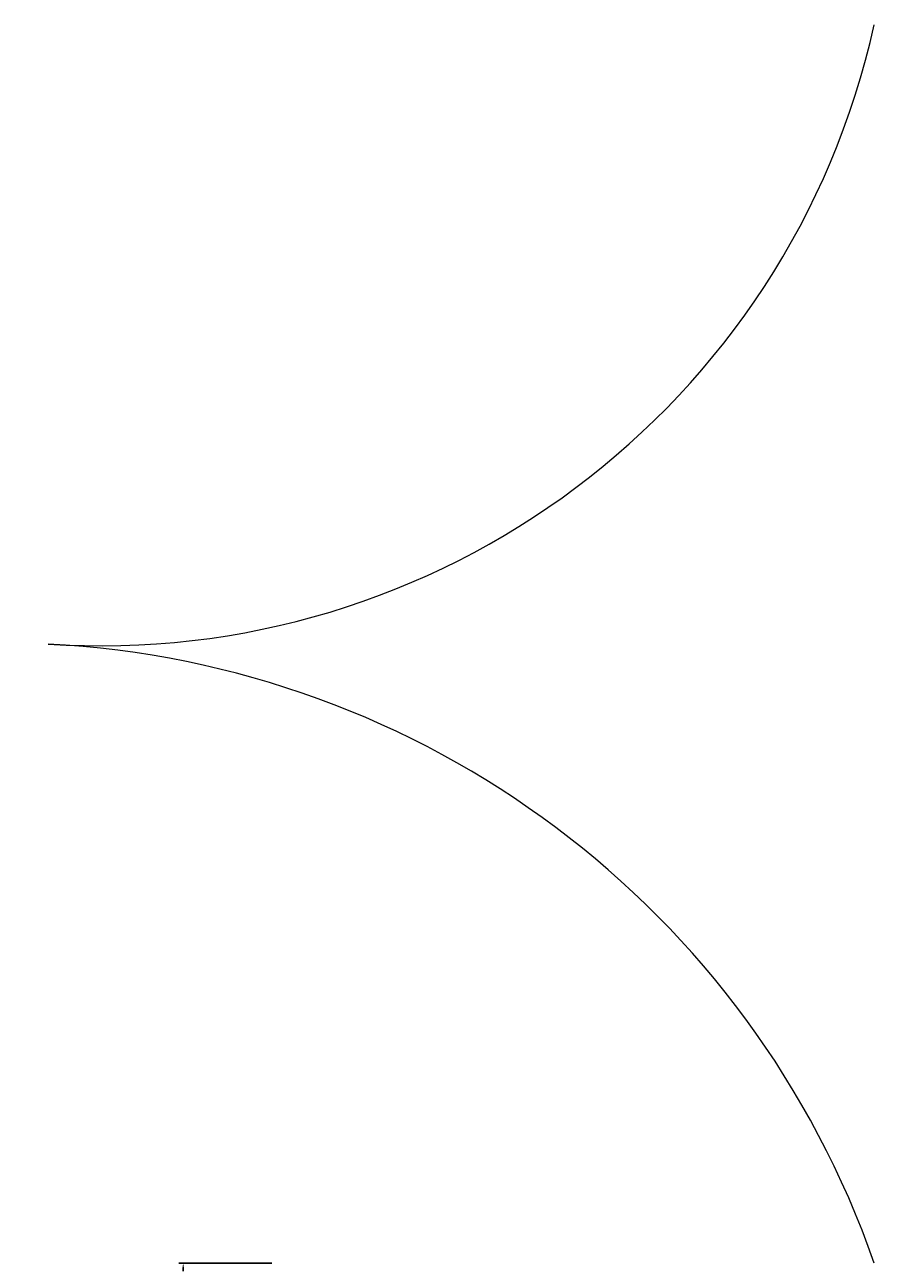
# Model space of a CAD drawing. Units: inches. Extents: x -86 to 2463, y -1058 to 68.
# Tile 9 of 17: x 15 to 49, y -273 to -223. Entities that reach past the tile are written whole.
import ezdxf

# ---------------------------------------------------------------- set-up
doc = ezdxf.new("R2010")
doc.units = ezdxf.units.IN
doc.header["$MEASUREMENT"] = 0
doc.layers.add('A-ANNO-DIMS', color=2, linetype='Continuous', lineweight=18)
doc.layers.add('A-DOOR', color=3, linetype='Continuous', lineweight=18)
doc.styles.get("Standard").update_dxf_attribs({"font": 'arial.ttf'})
doc.dimstyles.get("Standard").update_dxf_attribs({"dimtxt": 0.18, "dimasz": 0.18, "dimexe": 0.18, "dimexo": 0.0625, "dimgap": 0.09, "dimtad": 0, "dimtih": 1, "dimtoh": 1, "dimdec": 4, "dimzin": 0, "dimdsep": 46, "dimtxsty": 'Standard', "dimcen": 0.09, "dimadec": 0, "dimazin": 0, "dimtfac": 1, "dimtdec": 4, "dimtofl": 0, "dimtmove": 0, "dimatfit": 3, "dimfxl": 1, "dimtolj": 1, "dimtzin": 0, "dimarcsym": 0})

# ---------------------------------------------------------------- blocks, each defined once
blk = doc.blocks.new('*D11')
at = {"layer": 'A-ANNO-DIMS', "color": 0, "lineweight": -2, "transparency": 16777216}
for p, q in [((24.698, -272.574), (20.981, -272.574)), ((21.161, -272.754), (21.161, -272.894)), ((21.161, -273.394), (21.161, -273.254)), ((24.698, -273.574), (20.981, -273.574))]:
    blk.add_line(p, q, dxfattribs=at)
at = {"layer": 'A-ANNO-DIMS', "color": 0, "transparency": 16777216}
for points in [[(21.131, -272.754), (21.191, -272.754), (21.161, -272.574)], [(21.131, -273.394), (21.191, -273.394), (21.161, -273.574)]]:
    blk.add_solid(points, dxfattribs=at)
at = {"layer": 'Defpoints', "color": 0, "transparency": 16777216}
for p in [(24.761, -272.574), (21.161, -273.574), (24.761, -273.574)]:
    blk.add_point(p, dxfattribs=at)
at = {"layer": 'A-ANNO-DIMS', "color": 0, "transparency": 16777216, "insert": (21.161, -273.074), "char_height": 0.18, "attachment_point": 5}
blk.add_mtext('\\A1;1 TYP.', dxfattribs=at)
blk = doc.blocks.new('*D38')
at = {"layer": 'A-ANNO-DIMS', "color": 0, "lineweight": -2, "transparency": 16777216}
for p, q in [((15.698, -222.104), (-86.019, -222.104)), ((-85.839, -222.284), (-85.839, -247.657)), ((-85.839, -273.394), (-85.839, -248.021)), ((15.698, -273.574), (-86.019, -273.574))]:
    blk.add_line(p, q, dxfattribs=at)
at = {"layer": 'A-ANNO-DIMS', "color": 0, "transparency": 16777216}
for points in [[(-85.869, -222.284), (-85.809, -222.284), (-85.839, -222.104)], [(-85.869, -273.394), (-85.809, -273.394), (-85.839, -273.574)]]:
    blk.add_solid(points, dxfattribs=at)
at = {"layer": 'Defpoints', "color": 0, "transparency": 16777216}
for p in [(-85.839, -222.104), (15.761, -222.104), (15.761, -273.574)]:
    blk.add_point(p, dxfattribs=at)
at = {"layer": 'A-ANNO-DIMS', "color": 0, "transparency": 16777216, "insert": (-85.839, -247.839), "char_height": 0.18, "attachment_point": 5}
blk.add_mtext('\\A1;51.47', dxfattribs=at)

msp = doc.modelspace()

# ---------------------------------------------------------------- linework, layer by layer
at = {"layer": 'A-DOOR'}
for centre, radius, start, end in [((17.874, -216.278), 31.632, 266.1692, 347.5372), ((13.904, -284.698), 36.905, 19.178, 87.1156)]:
    msp.add_arc(centre, radius, start, end, dxfattribs=at)

# ---------------------------------------------------------------- dimensions: what is measured, and where the dimension line sits
at = {"layer": 'A-ANNO-DIMS'}
dim = msp.add_linear_dim(base=(-85.839, -222.104), p1=(15.761, -273.574), p2=(15.761, -222.104), angle=90, dimstyle='Standard', override={"dimdec": 2, "dimlfac": 1, "dimrnd": 0, "dimzin": 0, "dimdsep": 46, "dimlunit": 2}, dxfattribs=at)
dim.commit()
dim.dimension.update_dxf_attribs({"geometry": '*D38', "text_midpoint": (-85.839, -247.839)})
dim = msp.add_linear_dim(base=(21.161, -273.574), p1=(24.761, -272.574), p2=(24.761, -273.574), angle=270, text='<> TYP.', dimstyle='Standard', override={"dimdec": 0, "dimlfac": 1, "dimrnd": 0, "dimzin": 0, "dimdsep": 46, "dimlunit": 2}, dxfattribs=at)
dim.commit()
dim.dimension.update_dxf_attribs({"geometry": '*D11', "text_midpoint": (21.161, -273.074)})

doc.saveas('drawing.dxf')
